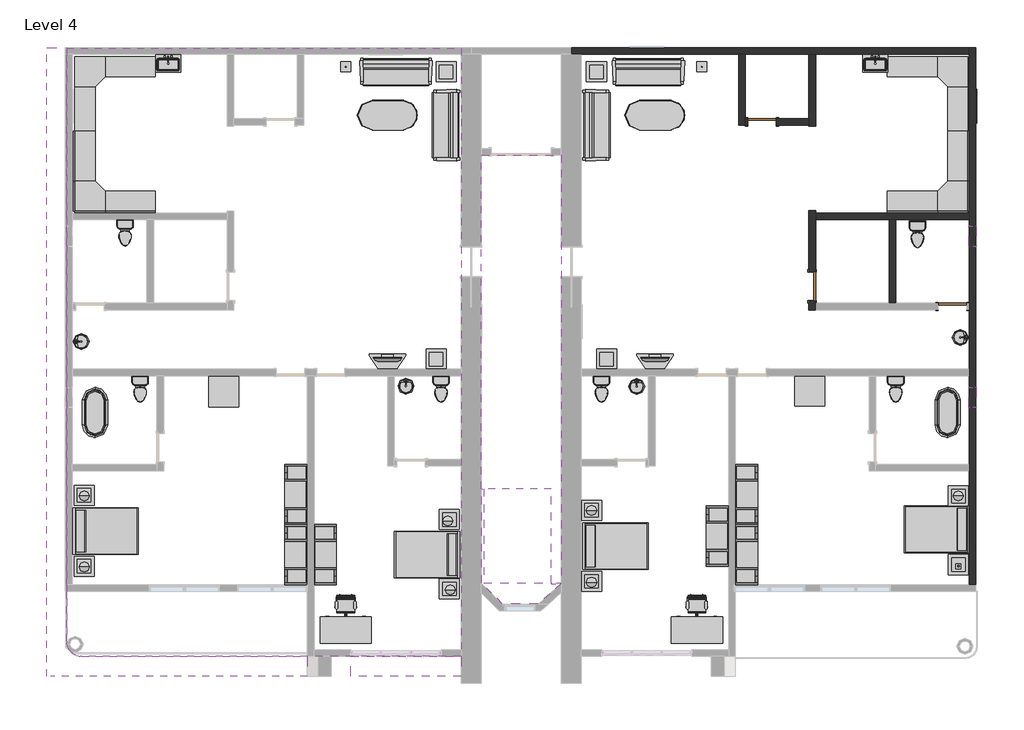
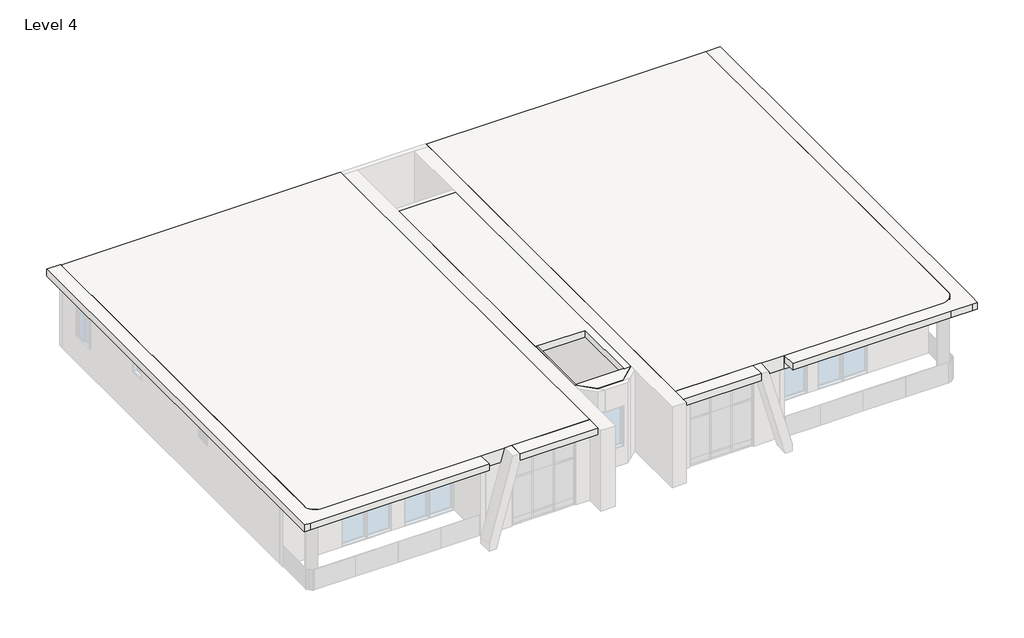
# One storey, part 3 of 3: 42 furniture elements, 14 flow terminals, 10 light fixtures, 8 walls, 5 slabs, 3 doors, 3 windows.
"""IFC4 building model written with IfcOpenShell, lengths in millimetres."""

from ifc_helpers import new_model, si_unit, point, frame, frame_2d, origin, place, context, project, spatial, polyline, circle_curve, trimmed, segment, composite_curve, outline, extrude, faceted_brep, transform, mapped, element, save
from components import door_2703ae13, door_10fd3a06, flow_terminal_38af2918, flow_terminal_d49f872f, toilet_domestic_3d_toilet_domestic_3d_f7549cf7, toilet_domestic_3d_toilet_domestic_3d_183bbd19, flow_terminal_b374fae2, furniture_07436f11, furniture_096e7f55, chair_task_arms_chair_task_arms_fa5a08ef, furniture_072f6425, furniture_cf0b6580, furniture_aff9b2fb, furniture_56245f3a, tv_stand_tv_stand_6ce107e5, furniture_b5c51a22, furniture_2c34a4f9, furniture_4d44e21c, furniture_45e3acac, light_fixture_100w_120v_8564026f, table_lamp_hemispheric_60w_120v_02721d88, window_0038ecf3, window_54100e87

model = new_model("IFC4")

# Units and contexts
model_context = context("Model", 3, world=origin())
ifc_project = project(units=[si_unit("LENGTHUNIT", "METRE", prefix="MILLI")], contexts=[model_context])

# Site, building, storey
site = spatial("IfcSite", under=ifc_project)
building = spatial("IfcBuilding", under=site)
storey = spatial("IfcBuildingStorey", under=building, Name="Level 4", Elevation=10972.8)

# Doors
placement = place(None, origin())
door_shape = door_2703ae13(model_context)
element("IfcDoor", 1, ObjectType="Door-Single-Panel.0001 : 34\" x 80\"", at=placement, inside=storey, context=model_context, shape_type="MappedRepresentation", body=[
    mapped(door_shape, transform((2522.0012296, 9464.0758558, 10972.8), x_axis=(-1.0, 0.0, 0.0), y_axis=(0.0, -1.0, 0.0), z_axis=(0.0, 0.0, 1.0))),
])
door_2_shape = door_10fd3a06(model_context)
element("IfcDoor", 2, ObjectType="Door-Single-Panel.0001 : 34\" x 80\"", at=placement, inside=storey, context=model_context, shape_type="MappedRepresentation", body=[
    mapped(door_2_shape, transform((8313.2012296, 3850.6758558, 10972.8), x_axis=(1.0, 0.0, 0.0), y_axis=(0.0, 1.0, 0.0), z_axis=(0.0, 0.0, 1.0))),
])
element("IfcDoor", 3, ObjectType="Door-Single-Panel.0001 : 34\" x 80\"", at=placement, inside=storey, context=model_context, shape_type="MappedRepresentation", body=[
    mapped(door_2_shape, transform((4046.0012296, 4460.2758558, 10972.8), x_axis=(0.0, -1.0, 0.0), y_axis=(1.0, 0.0, 0.0), z_axis=(0.0, 0.0, 1.0))),
])

# Flow terminals
flow_terminal_shape = flow_terminal_38af2918(model_context)
element("IfcFlowTerminal", 4, ObjectType="Sink Kitchen-Single : 30\" x 21\"", at=placement, inside=storey, context=model_context, shape_type="MappedRepresentation", body=[
    mapped(flow_terminal_shape, transform((-15540.388011, 11239.7304546, 10972.8), x_axis=(1.0, 0.0, 0.0), y_axis=(0.0, 1.0, 0.0), z_axis=(0.0, 0.0, 1.0))),
])
element("IfcFlowTerminal", 5, ObjectType="Sink Kitchen-Single : 30\" x 21\"", at=placement, inside=storey, context=model_context, shape_type="MappedRepresentation", body=[
    mapped(flow_terminal_shape, transform((5948.011989, 11239.7304546, 10972.8), x_axis=(1.0, 0.0, 0.0), y_axis=(0.0, 1.0, 0.0), z_axis=(0.0, 0.0, 1.0))),
])
flow_terminal_2_shape = flow_terminal_d49f872f(model_context)
element("IfcFlowTerminal", 6, ObjectType="Sink Vanity-Round : 19\" x 19\"", at=placement, inside=storey, context=model_context, shape_type="MappedRepresentation", body=[
    mapped(flow_terminal_2_shape, transform((-18084.6070794, 2687.2241152, 10972.8), x_axis=(0.0, 1.0, 0.0), y_axis=(-1.0, 0.0, 0.0), z_axis=(0.0, 0.0, 1.0))),
])
element("IfcFlowTerminal", 7, ObjectType="Sink Vanity-Round : 19\" x 19\"", at=placement, inside=storey, context=model_context, shape_type="MappedRepresentation", body=[
    mapped(flow_terminal_2_shape, transform((8462.2249463, 3007.5275963, 10972.8), x_axis=(0.0, -1.0, 0.0), y_axis=(1.0, 0.0, 0.0), z_axis=(0.0, 0.0, 1.0))),
])
element("IfcFlowTerminal", 8, ObjectType="Sink Vanity-Round : 19\" x 19\"", at=placement, inside=storey, context=model_context, shape_type="MappedRepresentation", body=[
    mapped(flow_terminal_2_shape, transform((-8395.050511, 1341.8921141, 10972.8), x_axis=(1.0, 0.0, 0.0), y_axis=(0.0, 1.0, 0.0), z_axis=(0.0, 0.0, 1.0))),
])
element("IfcFlowTerminal", 9, ObjectType="Sink Vanity-Round : 19\" x 19\"", at=placement, inside=storey, context=model_context, shape_type="MappedRepresentation", body=[
    mapped(flow_terminal_2_shape, transform((-1384.650511, 1331.0855344, 10972.8), x_axis=(1.0, 0.0, 0.0), y_axis=(0.0, 1.0, 0.0), z_axis=(0.0, 0.0, 1.0))),
])
toilet_domestic_3d_toilet_domestic_3d_shape = toilet_domestic_3d_toilet_domestic_3d_f7549cf7(model_context)
toilet_domestic_3d_toilet_domestic_3d_2_shape = toilet_domestic_3d_toilet_domestic_3d_183bbd19(model_context)
element("IfcFlowTerminal", 10, ObjectType="Toilet-Domestic-3D : Toilet-Domestic-3D", at=placement, inside=storey, context=model_context, shape_type="MappedRepresentation", body=[
    mapped(toilet_domestic_3d_toilet_domestic_3d_shape, transform((6586.0012296, 1247.7798284, 10972.8), x_axis=(1.0, 0.0, 0.0), y_axis=(0.0, 1.0, 0.0), z_axis=(0.0, 0.0, 1.0))),
    mapped(toilet_domestic_3d_toilet_domestic_3d_2_shape, transform((6586.0012296, 1247.7798284, 10972.8), x_axis=(1.0, 0.0, 0.0), y_axis=(0.0, 1.0, 0.0), z_axis=(0.0, 0.0, 1.0))),
])
element("IfcFlowTerminal", 11, ObjectType="Toilet-Domestic-3D : Toilet-Domestic-3D", at=placement, inside=storey, context=model_context, shape_type="MappedRepresentation", body=[
    mapped(toilet_domestic_3d_toilet_domestic_3d_shape, transform((-2354.7987704, 1247.7798284, 10972.8), x_axis=(1.0, 0.0, 0.0), y_axis=(0.0, 1.0, 0.0), z_axis=(0.0, 0.0, 1.0))),
    mapped(toilet_domestic_3d_toilet_domestic_3d_2_shape, transform((-2354.7987704, 1247.7798284, 10972.8), x_axis=(1.0, 0.0, 0.0), y_axis=(0.0, 1.0, 0.0), z_axis=(0.0, 0.0, 1.0))),
])
element("IfcFlowTerminal", 12, ObjectType="Toilet-Domestic-3D : Toilet-Domestic-3D", at=placement, inside=storey, context=model_context, shape_type="MappedRepresentation", body=[
    mapped(toilet_domestic_3d_toilet_domestic_3d_shape, transform((-16375.5987704, 1247.7798284, 10972.8), x_axis=(1.0, 0.0, 0.0), y_axis=(0.0, 1.0, 0.0), z_axis=(0.0, 0.0, 1.0))),
    mapped(toilet_domestic_3d_toilet_domestic_3d_2_shape, transform((-16375.5987704, 1247.7798284, 10972.8), x_axis=(1.0, 0.0, 0.0), y_axis=(0.0, 1.0, 0.0), z_axis=(0.0, 0.0, 1.0))),
])
element("IfcFlowTerminal", 13, ObjectType="Toilet-Domestic-3D : Toilet-Domestic-3D", at=placement, inside=storey, context=model_context, shape_type="MappedRepresentation", body=[
    mapped(toilet_domestic_3d_toilet_domestic_3d_shape, transform((-16832.7987704, 5997.5798284, 10972.8), x_axis=(1.0, 0.0, 0.0), y_axis=(0.0, 1.0, 0.0), z_axis=(0.0, 0.0, 1.0))),
    mapped(toilet_domestic_3d_toilet_domestic_3d_2_shape, transform((-16832.7987704, 5997.5798284, 10972.8), x_axis=(1.0, 0.0, 0.0), y_axis=(0.0, 1.0, 0.0), z_axis=(0.0, 0.0, 1.0))),
])
element("IfcFlowTerminal", 14, ObjectType="Toilet-Domestic-3D : Toilet-Domestic-3D", at=placement, inside=storey, context=model_context, shape_type="MappedRepresentation", body=[
    mapped(toilet_domestic_3d_toilet_domestic_3d_shape, transform((7246.4012296, 5946.7798284, 10972.8), x_axis=(1.0, 0.0, 0.0), y_axis=(0.0, 1.0, 0.0), z_axis=(0.0, 0.0, 1.0))),
    mapped(toilet_domestic_3d_toilet_domestic_3d_2_shape, transform((7246.4012296, 5946.7798284, 10972.8), x_axis=(1.0, 0.0, 0.0), y_axis=(0.0, 1.0, 0.0), z_axis=(0.0, 0.0, 1.0))),
])
element("IfcFlowTerminal", 15, ObjectType="Toilet-Domestic-3D : Toilet-Domestic-3D", at=placement, inside=storey, context=model_context, shape_type="MappedRepresentation", body=[
    mapped(toilet_domestic_3d_toilet_domestic_3d_shape, transform((-7231.5987704, 1247.7798284, 10972.8), x_axis=(1.0, 0.0, 0.0), y_axis=(0.0, 1.0, 0.0), z_axis=(0.0, 0.0, 1.0))),
    mapped(toilet_domestic_3d_toilet_domestic_3d_2_shape, transform((-7231.5987704, 1247.7798284, 10972.8), x_axis=(1.0, 0.0, 0.0), y_axis=(0.0, 1.0, 0.0), z_axis=(0.0, 0.0, 1.0))),
])
flow_terminal_3_shape = flow_terminal_b374fae2(model_context)
element("IfcFlowTerminal", 16, ObjectType="Tub-Free Standing-3D : 30\" x 60\"", at=placement, inside=storey, context=model_context, shape_type="MappedRepresentation", body=[
    mapped(flow_terminal_3_shape, transform((-17747.1987704, 624.8758558, 10972.8), x_axis=(1.0, 0.0, 0.0), y_axis=(0.0, 1.0, 0.0), z_axis=(0.0, 0.0, 1.0))),
])
element("IfcFlowTerminal", 17, ObjectType="Tub-Free Standing-3D : 30\" x 60\"", at=placement, inside=storey, context=model_context, shape_type="MappedRepresentation", body=[
    mapped(flow_terminal_3_shape, transform((8160.8012296, 624.8758558, 10972.8), x_axis=(1.0, 0.0, 0.0), y_axis=(0.0, 1.0, 0.0), z_axis=(0.0, 0.0, 1.0))),
])

# Furniture
furniture_shape = furniture_07436f11(model_context)
element("IfcFurniture", 18, ObjectType="96\" x 96\"", at=placement, inside=storey, context=model_context, shape_type="MappedRepresentation", body=[
    mapped(furniture_shape, transform((-18275.8670182, 11991.0988634, 10972.8), x_axis=(1.0, 0.0, 0.0), y_axis=(0.0, 1.0, 0.0), z_axis=(0.0, 0.0, 1.0))),
])
element("IfcFurniture", 19, ObjectType="96\" x 96\"", at=placement, inside=storey, context=model_context, shape_type="MappedRepresentation", body=[
    mapped(furniture_shape, transform((9316.2242372, 11364.3441035, 10972.8), x_axis=(0.0, -1.0, 0.0), y_axis=(1.0, 0.0, 0.0), z_axis=(0.0, 0.0, 1.0))),
])
furniture_2_shape = furniture_096e7f55(model_context)
element("IfcFurniture", 20, ObjectType="Bed-Shaker : Double 56\" x 78\"", at=placement, inside=storey, context=model_context, shape_type="MappedRepresentation", body=[
    mapped(furniture_2_shape, transform((-18407.5987704, -2962.8741442, 10972.8), x_axis=(0.0, 1.0, 0.0), y_axis=(-1.0, 0.0, 0.0), z_axis=(0.0, 0.0, 1.0))),
])
element("IfcFurniture", 21, ObjectType="Bed-Shaker : Double 56\" x 78\"", at=placement, inside=storey, context=model_context, shape_type="MappedRepresentation", body=[
    mapped(furniture_2_shape, transform((-6672.7987704, -3712.1741442, 10972.8), x_axis=(0.0, -1.0, 0.0), y_axis=(1.0, 0.0, 0.0), z_axis=(0.0, 0.0, 1.0))),
])
element("IfcFurniture", 22, ObjectType="Bed-Shaker : Double 56\" x 78\"", at=placement, inside=storey, context=model_context, shape_type="MappedRepresentation", body=[
    mapped(furniture_2_shape, transform((-2913.5987704, -3420.0741442, 10972.8), x_axis=(0.0, 1.0, 0.0), y_axis=(-1.0, 0.0, 0.0), z_axis=(0.0, 0.0, 1.0))),
])
element("IfcFurniture", 23, ObjectType="Bed-Shaker : Double 56\" x 78\"", at=placement, inside=storey, context=model_context, shape_type="MappedRepresentation", body=[
    mapped(furniture_2_shape, transform((8821.2012296, -2950.1741442, 10972.8), x_axis=(0.0, -1.0, 0.0), y_axis=(1.0, 0.0, 0.0), z_axis=(0.0, 0.0, 1.0))),
])
chair_task_arms_chair_task_arms_shape = chair_task_arms_chair_task_arms_fa5a08ef(model_context)
element("IfcFurniture", 24, ObjectType="Chair-Task Arms : Chair-Task Arms", at=placement, inside=storey, context=model_context, shape_type="MappedRepresentation", body=[
    mapped(chair_task_arms_chair_task_arms_shape, transform((681.7920493, -5184.3566833, 10972.8), x_axis=(-1.0, 0.0, 0.0), y_axis=(0.0, -1.0, 0.0), z_axis=(0.0, 0.0, 1.0))),
])
element("IfcFurniture", 25, ObjectType="Chair-Task Arms : Chair-Task Arms", at=placement, inside=storey, context=model_context, shape_type="MappedRepresentation", body=[
    mapped(chair_task_arms_chair_task_arms_shape, transform((-9986.2079507, -5184.3566833, 10972.8), x_axis=(-1.0, 0.0, 0.0), y_axis=(0.0, -1.0, 0.0), z_axis=(0.0, 0.0, 1.0))),
])
furniture_3_shape = furniture_072f6425(model_context)
element("IfcFurniture", 26, ObjectType="Desk : 60\" x 30\"", at=placement, inside=storey, context=model_context, shape_type="MappedRepresentation", body=[
    mapped(furniture_3_shape, transform((-10889.1987704, -6371.702585, 10972.8), x_axis=(1.0, 0.0, 0.0), y_axis=(0.0, 1.0, 0.0), z_axis=(0.0, 0.0, 1.0))),
])
element("IfcFurniture", 27, ObjectType="Desk : 60\" x 30\"", at=placement, inside=storey, context=model_context, shape_type="MappedRepresentation", body=[
    mapped(furniture_3_shape, transform((-221.1987704, -6371.702585, 10972.8), x_axis=(1.0, 0.0, 0.0), y_axis=(0.0, 1.0, 0.0), z_axis=(0.0, 0.0, 1.0))),
])
furniture_4_shape = furniture_cf0b6580(model_context)
element("IfcFurniture", 28, ObjectType="Entertainment Center : 72\" x 72\" x 24\"", at=placement, inside=storey, context=model_context, shape_type="MappedRepresentation", body=[
    mapped(furniture_4_shape, transform((1607.6012296, -3134.3241442, 10972.8), x_axis=(0.0, -1.0, 0.0), y_axis=(1.0, 0.0, 0.0), z_axis=(0.0, 0.0, 1.0))),
])
element("IfcFurniture", 29, ObjectType="Entertainment Center : 72\" x 72\" x 24\"", at=placement, inside=storey, context=model_context, shape_type="MappedRepresentation", body=[
    mapped(furniture_4_shape, transform((1607.6012296, -3693.1241442, 10972.8), x_axis=(0.0, 1.0, 0.0), y_axis=(-1.0, 0.0, 0.0), z_axis=(0.0, 0.0, 1.0))),
])
element("IfcFurniture", 30, ObjectType="Entertainment Center : 72\" x 72\" x 24\"", at=placement, inside=storey, context=model_context, shape_type="MappedRepresentation", body=[
    mapped(furniture_4_shape, transform((1607.6012296, -1864.3241442, 10972.8), x_axis=(0.0, 1.0, 0.0), y_axis=(-1.0, 0.0, 0.0), z_axis=(0.0, 0.0, 1.0))),
])
element("IfcFurniture", 31, ObjectType="Entertainment Center : 72\" x 72\" x 24\"", at=placement, inside=storey, context=model_context, shape_type="MappedRepresentation", body=[
    mapped(furniture_4_shape, transform((-11193.9987704, -3693.1241442, 10972.8), x_axis=(0.0, -1.0, 0.0), y_axis=(1.0, 0.0, 0.0), z_axis=(0.0, 0.0, 1.0))),
])
element("IfcFurniture", 32, ObjectType="Entertainment Center : 72\" x 72\" x 24\"", at=placement, inside=storey, context=model_context, shape_type="MappedRepresentation", body=[
    mapped(furniture_4_shape, transform((-11193.9987704, -1864.3241442, 10972.8), x_axis=(0.0, -1.0, 0.0), y_axis=(1.0, 0.0, 0.0), z_axis=(0.0, 0.0, 1.0))),
])
element("IfcFurniture", 33, ObjectType="Entertainment Center : 72\" x 72\" x 24\"", at=placement, inside=storey, context=model_context, shape_type="MappedRepresentation", body=[
    mapped(furniture_4_shape, transform((-11193.9987704, -3693.1241442, 10972.8), x_axis=(0.0, 1.0, 0.0), y_axis=(-1.0, 0.0, 0.0), z_axis=(0.0, 0.0, 1.0))),
])
furniture_5_shape = furniture_aff9b2fb(model_context)
element("IfcFurniture", 34, ObjectType="Sofa-Pensi : 84\"", at=placement, inside=storey, context=model_context, shape_type="MappedRepresentation", body=[
    mapped(furniture_5_shape, transform((-8881.8050204, 10710.9660197, 10972.8), x_axis=(1.0, 0.0, 0.0), y_axis=(0.0, 1.0, 0.0), z_axis=(0.0, 0.0, 1.0))),
])
element("IfcFurniture", 35, ObjectType="Sofa-Pensi : 84\"", at=placement, inside=storey, context=model_context, shape_type="MappedRepresentation", body=[
    mapped(furniture_5_shape, transform((-7356.3086065, 9641.0821058, 10972.8), x_axis=(0.0, -1.0, 0.0), y_axis=(1.0, 0.0, 0.0), z_axis=(0.0, 0.0, 1.0))),
])
element("IfcFurniture", 36, ObjectType="Sofa-Pensi : 84\"", at=placement, inside=storey, context=model_context, shape_type="MappedRepresentation", body=[
    mapped(furniture_5_shape, transform((-2230.0889343, 9083.8696058, 10972.8), x_axis=(0.0, 1.0, 0.0), y_axis=(-1.0, 0.0, 0.0), z_axis=(0.0, 0.0, 1.0))),
])
element("IfcFurniture", 37, ObjectType="Sofa-Pensi : 84\"", at=placement, inside=storey, context=model_context, shape_type="MappedRepresentation", body=[
    mapped(furniture_5_shape, transform((-1211.0050204, 10710.9660197, 10972.8), x_axis=(1.0, 0.0, 0.0), y_axis=(0.0, 1.0, 0.0), z_axis=(0.0, 0.0, 1.0))),
])
furniture_6_shape = furniture_56245f3a(model_context)
element("IfcFurniture", 38, ObjectType="TV - Flat Screen : 32\"", at=placement, inside=storey, context=model_context, shape_type="MappedRepresentation", body=[
    mapped(furniture_6_shape, transform((-8861.1432846, 2232.8144794, 11887.2), x_axis=(-1.0, 0.0, 0.0), y_axis=(0.0, -1.0, 0.0), z_axis=(0.0, 0.0, 1.0))),
])
element("IfcFurniture", 39, ObjectType="TV - Flat Screen : 32\"", at=placement, inside=storey, context=model_context, shape_type="MappedRepresentation", body=[
    mapped(furniture_6_shape, transform((-733.1432846, 2232.8144794, 11887.2), x_axis=(-1.0, 0.0, 0.0), y_axis=(0.0, -1.0, 0.0), z_axis=(0.0, 0.0, 1.0))),
])
tv_stand_tv_stand_shape = tv_stand_tv_stand_6ce107e5(model_context)
element("IfcFurniture", 40, ObjectType="TV Stand : TV Stand", at=placement, inside=storey, context=model_context, shape_type="MappedRepresentation", body=[
    mapped(tv_stand_tv_stand_shape, transform((-8732.0107683, 1945.6758558, 10972.8), x_axis=(-1.0, 0.0, 0.0), y_axis=(0.0, -1.0, 0.0), z_axis=(0.0, 0.0, 1.0))),
])
element("IfcFurniture", 41, ObjectType="TV Stand : TV Stand", at=placement, inside=storey, context=model_context, shape_type="MappedRepresentation", body=[
    mapped(tv_stand_tv_stand_shape, transform((-604.0107683, 1945.6758558, 10972.8), x_axis=(-1.0, 0.0, 0.0), y_axis=(0.0, -1.0, 0.0), z_axis=(0.0, 0.0, 1.0))),
])
furniture_7_shape = furniture_b5c51a22(model_context)
element("IfcFurniture", 42, ObjectType="Table-Coffee : 24\" x 24\" x 24\"", at=placement, inside=storey, context=model_context, shape_type="MappedRepresentation", body=[
    mapped(furniture_7_shape, transform((-7097.4645371, 10892.864778, 10972.8), x_axis=(1.0, 0.0, 0.0), y_axis=(0.0, 1.0, 0.0), z_axis=(0.0, 0.0, 1.0))),
])
element("IfcFurniture", 43, ObjectType="Table-Coffee : 24\" x 24\" x 24\"", at=placement, inside=storey, context=model_context, shape_type="MappedRepresentation", body=[
    mapped(furniture_7_shape, transform((-2525.4645371, 10892.864778, 10972.8), x_axis=(1.0, 0.0, 0.0), y_axis=(0.0, 1.0, 0.0), z_axis=(0.0, 0.0, 1.0))),
])
element("IfcFurniture", 44, ObjectType="Table-Coffee : 24\" x 24\" x 24\"", at=placement, inside=storey, context=model_context, shape_type="MappedRepresentation", body=[
    mapped(furniture_7_shape, transform((-7402.2645371, 2155.264778, 10972.8), x_axis=(1.0, 0.0, 0.0), y_axis=(0.0, 1.0, 0.0), z_axis=(0.0, 0.0, 1.0))),
])
element("IfcFurniture", 45, ObjectType="Table-Coffee : 24\" x 24\" x 24\"", at=placement, inside=storey, context=model_context, shape_type="MappedRepresentation", body=[
    mapped(furniture_7_shape, transform((-2220.6645371, 2155.264778, 10972.8), x_axis=(1.0, 0.0, 0.0), y_axis=(0.0, 1.0, 0.0), z_axis=(0.0, 0.0, 1.0))),
])
element("IfcFurniture", 46, ObjectType="Table-Coffee : 24\" x 24\" x 24\"", at=placement, inside=storey, context=model_context, shape_type="MappedRepresentation", body=[
    mapped(furniture_7_shape, transform((-2677.8645371, -4601.135222, 10972.8), x_axis=(1.0, 0.0, 0.0), y_axis=(0.0, 1.0, 0.0), z_axis=(0.0, 0.0, 1.0))),
])
element("IfcFurniture", 47, ObjectType="Table-Coffee : 24\" x 24\" x 24\"", at=placement, inside=storey, context=model_context, shape_type="MappedRepresentation", body=[
    mapped(furniture_7_shape, transform((-18095.6645371, -4143.935222, 10972.8), x_axis=(1.0, 0.0, 0.0), y_axis=(0.0, 1.0, 0.0), z_axis=(0.0, 0.0, 1.0))),
])
element("IfcFurniture", 48, ObjectType="Table-Coffee : 24\" x 24\" x 24\"", at=placement, inside=storey, context=model_context, shape_type="MappedRepresentation", body=[
    mapped(furniture_7_shape, transform((-18095.6645371, -1984.935222, 10972.8), x_axis=(1.0, 0.0, 0.0), y_axis=(0.0, 1.0, 0.0), z_axis=(0.0, 0.0, 1.0))),
])
element("IfcFurniture", 49, ObjectType="Table-Coffee : 24\" x 24\" x 24\"", at=placement, inside=storey, context=model_context, shape_type="MappedRepresentation", body=[
    mapped(furniture_7_shape, transform((-2677.8645371, -2442.135222, 10972.8), x_axis=(1.0, 0.0, 0.0), y_axis=(0.0, 1.0, 0.0), z_axis=(0.0, 0.0, 1.0))),
])
element("IfcFurniture", 50, ObjectType="Table-Coffee : 24\" x 24\" x 24\"", at=placement, inside=storey, context=model_context, shape_type="MappedRepresentation", body=[
    mapped(furniture_7_shape, transform((8472.7354629, -4093.135222, 10972.8), x_axis=(1.0, 0.0, 0.0), y_axis=(0.0, 1.0, 0.0), z_axis=(0.0, 0.0, 1.0))),
])
element("IfcFurniture", 51, ObjectType="Table-Coffee : 24\" x 24\" x 24\"", at=placement, inside=storey, context=model_context, shape_type="MappedRepresentation", body=[
    mapped(furniture_7_shape, transform((8472.7354629, -2010.335222, 10972.8), x_axis=(1.0, 0.0, 0.0), y_axis=(0.0, 1.0, 0.0), z_axis=(0.0, 0.0, 1.0))),
])
element("IfcFurniture", 52, ObjectType="Table-Coffee : 24\" x 24\" x 24\"", at=placement, inside=storey, context=model_context, shape_type="MappedRepresentation", body=[
    mapped(furniture_7_shape, transform((-6995.8645371, -4832.0414601, 10972.8), x_axis=(1.0, 0.0, 0.0), y_axis=(0.0, 1.0, 0.0), z_axis=(0.0, 0.0, 1.0))),
])
element("IfcFurniture", 53, ObjectType="Table-Coffee : 24\" x 24\" x 24\"", at=placement, inside=storey, context=model_context, shape_type="MappedRepresentation", body=[
    mapped(furniture_7_shape, transform((-6995.8645371, -2723.8414601, 10972.8), x_axis=(1.0, 0.0, 0.0), y_axis=(0.0, 1.0, 0.0), z_axis=(0.0, 0.0, 1.0))),
])
furniture_8_shape = furniture_2c34a4f9(model_context)
element("IfcFurniture", 54, ObjectType="Table-Dining Oval : 36\" x 72\"", at=placement, inside=storey, context=model_context, shape_type="MappedRepresentation", body=[
    mapped(furniture_8_shape, transform((-8455.3790983, 10025.3742164, 10972.8), x_axis=(1.0, 0.0, 0.0), y_axis=(0.0, 1.0, 0.0), z_axis=(0.0, 0.0, 1.0))),
])
element("IfcFurniture", 55, ObjectType="Table-Dining Oval : 36\" x 72\"", at=placement, inside=storey, context=model_context, shape_type="MappedRepresentation", body=[
    mapped(furniture_8_shape, transform((-327.3790983, 10025.3742164, 10972.8), x_axis=(1.0, 0.0, 0.0), y_axis=(0.0, 1.0, 0.0), z_axis=(0.0, 0.0, 1.0))),
])
furniture_9_shape = furniture_4d44e21c(model_context)
element("IfcFurniture", 56, ObjectType="Table-Rectangular : 36\" x 36\"", at=placement, inside=storey, context=model_context, shape_type="MappedRepresentation", body=[
    mapped(furniture_9_shape, transform((-13835.5987704, 1259.8758558, 10972.8), x_axis=(1.0, 0.0, 0.0), y_axis=(0.0, 1.0, 0.0), z_axis=(0.0, 0.0, 1.0))),
])
element("IfcFurniture", 57, ObjectType="Table-Rectangular : 36\" x 36\"", at=placement, inside=storey, context=model_context, shape_type="MappedRepresentation", body=[
    mapped(furniture_9_shape, transform((3969.8012296, 1285.2758558, 10972.8), x_axis=(1.0, 0.0, 0.0), y_axis=(0.0, 1.0, 0.0), z_axis=(0.0, 0.0, 1.0))),
])
furniture_10_shape = furniture_45e3acac(model_context)
element("IfcFurniture", 58, ObjectType="Work Station Cubicle : 96\" x 96\"", at=placement, inside=storey, context=model_context, shape_type="MappedRepresentation", body=[
    mapped(furniture_10_shape, transform((-18902.621778, 6827.207608, 10972.8), x_axis=(0.0, 1.0, 0.0), y_axis=(-1.0, 0.0, 0.0), z_axis=(0.0, 0.0, 1.0))),
])
element("IfcFurniture", 59, ObjectType="Work Station Cubicle : 96\" x 96\"", at=placement, inside=storey, context=model_context, shape_type="MappedRepresentation", body=[
    mapped(furniture_10_shape, transform((8689.4694774, 6200.4528481, 10972.8), x_axis=(-1.0, 0.0, 0.0), y_axis=(0.0, -1.0, 0.0), z_axis=(0.0, 0.0, 1.0))),
])

# Light fixtures
light_fixture_100w_120v_shape = light_fixture_100w_120v_8564026f(model_context)
element("IfcLightFixture", 60, ObjectType="100W - 120V", at=placement, inside=storey, context=model_context, shape_type="MappedRepresentation", body=[
    mapped(light_fixture_100w_120v_shape, transform((-10127.1987704, 11140.4758558, 10972.8), x_axis=(1.0, 0.0, 0.0), y_axis=(0.0, 1.0, 0.0), z_axis=(0.0, 0.0, 1.0))),
])
element("IfcLightFixture", 61, ObjectType="100W - 120V", at=placement, inside=storey, context=model_context, shape_type="MappedRepresentation", body=[
    mapped(light_fixture_100w_120v_shape, transform((693.2012296, 11140.4758558, 10972.8), x_axis=(1.0, 0.0, 0.0), y_axis=(0.0, 1.0, 0.0), z_axis=(0.0, 0.0, 1.0))),
])
table_lamp_hemispheric_60w_120v_shape = table_lamp_hemispheric_60w_120v_02721d88(model_context)
element("IfcLightFixture", 62, ObjectType="Table Lamp - Hemispheric : 60W - 120V", at=placement, inside=storey, context=model_context, shape_type="MappedRepresentation", body=[
    mapped(table_lamp_hemispheric_60w_120v_shape, transform((-18077.3987704, -1915.1241442, 11582.4), x_axis=(1.0, 0.0, 0.0), y_axis=(0.0, 1.0, 0.0), z_axis=(0.0, 0.0, 1.0))),
])
element("IfcLightFixture", 63, ObjectType="Table Lamp - Hemispheric : 60W - 120V", at=placement, inside=storey, context=model_context, shape_type="MappedRepresentation", body=[
    mapped(table_lamp_hemispheric_60w_120v_shape, transform((-7028.3987704, -2666.7303823, 11582.4), x_axis=(1.0, 0.0, 0.0), y_axis=(0.0, 1.0, 0.0), z_axis=(0.0, 0.0, 1.0))),
])
element("IfcLightFixture", 64, ObjectType="Table Lamp - Hemispheric : 60W - 120V", at=placement, inside=storey, context=model_context, shape_type="MappedRepresentation", body=[
    mapped(table_lamp_hemispheric_60w_120v_shape, transform((-2659.5987704, -2346.9241442, 11582.4), x_axis=(1.0, 0.0, 0.0), y_axis=(0.0, 1.0, 0.0), z_axis=(0.0, 0.0, 1.0))),
])
element("IfcLightFixture", 65, ObjectType="Table Lamp - Hemispheric : 60W - 120V", at=placement, inside=storey, context=model_context, shape_type="MappedRepresentation", body=[
    mapped(table_lamp_hemispheric_60w_120v_shape, transform((8491.0012296, -4048.7241442, 11887.2), x_axis=(1.0, 0.0, 0.0), y_axis=(0.0, 1.0, 0.0), z_axis=(0.0, 0.0, 1.0))),
])
element("IfcLightFixture", 66, ObjectType="Table Lamp - Hemispheric : 60W - 120V", at=placement, inside=storey, context=model_context, shape_type="MappedRepresentation", body=[
    mapped(table_lamp_hemispheric_60w_120v_shape, transform((8491.0012296, -1915.1241442, 11582.4), x_axis=(1.0, 0.0, 0.0), y_axis=(0.0, 1.0, 0.0), z_axis=(0.0, 0.0, 1.0))),
])
element("IfcLightFixture", 67, ObjectType="Table Lamp - Hemispheric : 60W - 120V", at=placement, inside=storey, context=model_context, shape_type="MappedRepresentation", body=[
    mapped(table_lamp_hemispheric_60w_120v_shape, transform((-2659.5987704, -4531.3241442, 11582.4), x_axis=(1.0, 0.0, 0.0), y_axis=(0.0, 1.0, 0.0), z_axis=(0.0, 0.0, 1.0))),
])
element("IfcLightFixture", 68, ObjectType="Table Lamp - Hemispheric : 60W - 120V", at=placement, inside=storey, context=model_context, shape_type="MappedRepresentation", body=[
    mapped(table_lamp_hemispheric_60w_120v_shape, transform((-6952.1987704, -4762.2303823, 11582.4), x_axis=(1.0, 0.0, 0.0), y_axis=(0.0, 1.0, 0.0), z_axis=(0.0, 0.0, 1.0))),
])
element("IfcLightFixture", 69, ObjectType="Table Lamp - Hemispheric : 60W - 120V", at=placement, inside=storey, context=model_context, shape_type="MappedRepresentation", body=[
    mapped(table_lamp_hemispheric_60w_120v_shape, transform((-18077.3987704, -4074.1241442, 11582.4), x_axis=(1.0, 0.0, 0.0), y_axis=(0.0, 1.0, 0.0), z_axis=(0.0, 0.0, 1.0))),
])

# Slabs
element("IfcSlab", 70, ObjectType="Generic - 12\" cream", at=placement, inside=storey, context=model_context, shape_type="SweptSolid", body=[
    extrude(outline(composite_curve([segment(polyline([(-6621.9987704, 11699.2758558), (-6621.9987704, -6791.9241442), (-11295.5987704, -6791.9241442), (-18153.5987704, -6791.9241442)]), True, "CONTINUOUS"), segment(trimmed(circle_curve(frame_2d((-18153.5987704, -6334.7241442)), 457.2), [point((-18153.5987704, -6791.9241442))], [point((-18610.7987704, -6334.7241442))], False, "CARTESIAN"), True, "CONTINUOUS"), segment(polyline([(-18610.7987704, -6334.7241442), (-18610.7987704, 11699.2758558), (-6621.9987704, 11699.2758558)]), True, "CONTINUOUS")], self_intersect=False)), frame((0.0, 0.0, 14020.8), z_axis=(0.0, 0.0, 1.0), x_axis=(1.0, 0.0, 0.0)), (0.0, 0.0, 1.0), 609.6),
    extrude(outline(composite_curve([segment(trimmed(circle_curve(frame_2d((8511.8043381, -6277.3874522)), 514.536692), [point((9024.4012296, -6322.0241442))], [point((8511.8043381, -6791.9241442))], False, "CARTESIAN"), True, "CONTINUOUS"), segment(polyline([(8511.8043381, -6791.9241442), (1709.2012296, -6791.9241442), (-2862.7987704, -6791.9241442), (-2964.3987704, -6791.9241442), (-2964.3987704, 11699.2758558), (9024.4012296, 11699.2758558), (9024.4012296, -6322.0241442)]), True, "CONTINUOUS")], self_intersect=False)), frame((0.0, 0.0, 14020.8), z_axis=(0.0, 0.0, 1.0), x_axis=(1.0, 0.0, 0.0)), (0.0, 0.0, 1.0), 609.6),
])
element("IfcSlab", 71, ObjectType="Generic - 12\" white", at=placement, inside=storey, context=model_context, shape_type="SweptSolid", body=[
    extrude(outline(composite_curve([segment(polyline([(9634.0012296, 11699.2758558), (9634.0012296, -6931.6241442), (9634.0012296, -7401.5241442), (9430.8012296, -7401.5241442), (8511.8043381, -7401.5241442), (1709.2012296, -7401.5241442), (1709.2012296, -6791.9241442), (8511.8043381, -6791.9241442)]), True, "CONTINUOUS"), segment(trimmed(circle_curve(frame_2d((8511.8043381, -6277.3874522)), 514.536692), [point((8511.8043381, -6791.9241442))], [point((9024.4012296, -6322.0241442))], True, "CARTESIAN"), True, "CONTINUOUS"), segment(polyline([(9024.4012296, -6322.0241442), (9024.4012296, 11699.2758558), (9634.0012296, 11699.2758558)]), True, "CONTINUOUS")], self_intersect=False)), frame((0.0, 0.0, 14325.6), z_axis=(0.0, 0.0, 1.0), x_axis=(1.0, 0.0, 0.0)), (0.0, 0.0, 1.0), 304.8),
    extrude(outline(composite_curve([segment(polyline([(-18610.7987704, 11724.6758558), (-18610.7987704, -6334.7241442)]), True, "CONTINUOUS"), segment(trimmed(circle_curve(frame_2d((-18153.5987704, -6334.7241442)), 457.2), [point((-18610.7987704, -6334.7241442))], [point((-18153.5987704, -6791.9241442))], True, "CARTESIAN"), True, "CONTINUOUS"), segment(polyline([(-18153.5987704, -6791.9241442), (-11295.5987704, -6791.9241442), (-11295.5987704, -7401.5241442), (-18966.3987704, -7401.5241442), (-19220.3987704, -7401.5241442), (-19220.3987704, 11724.6758558), (-18610.7987704, 11724.6758558)]), True, "CONTINUOUS")], self_intersect=False)), frame((0.0, 0.0, 14325.6), z_axis=(0.0, 0.0, 1.0), x_axis=(1.0, 0.0, 0.0)), (0.0, 0.0, 1.0), 304.8),
])
element("IfcSlab", 72, ObjectType="Generic - 12\" white", at=placement, inside=storey, context=model_context, shape_type="SweptSolid", body=[
    extrude(outline(polyline([(385.6468143, -6791.9241442), (385.6468143, -7401.5241442), (-2964.3987704, -7401.5241442), (-2964.3987704, -6791.9241442), (385.6468143, -6791.9241442)])), frame((0.0, 0.0, 14325.6), z_axis=(0.0, 0.0, 1.0), x_axis=(1.0, 0.0, 0.0)), (0.0, 0.0, 1.0), 304.8),
    extrude(outline(polyline([(-9974.7987704, -6791.9241442), (-6621.9987704, -6791.9241442), (-6621.9987704, -7401.5241442), (-9974.7987704, -7401.5241442), (-9974.7987704, -6791.9241442)])), frame((0.0, 0.0, 14325.6), z_axis=(0.0, 0.0, 1.0), x_axis=(1.0, 0.0, 0.0)), (0.0, 0.0, 1.0), 304.8),
])
element("IfcSlab", 73, ObjectType="Generic - 12\" white", at=placement, inside=storey, context=model_context, shape_type="SweptSolid", body=[
    extrude(outline(polyline([(-3573.9987704, 8448.0758558), (-3573.9987704, -1691.5549149), (-3573.9987704, -4572.9908503), (-3878.7987704, -4572.9908503), (-3878.7987704, -1691.5549149), (-6012.3987704, -1691.5549149), (-6012.3987704, 8448.0758558), (-3573.9987704, 8448.0758558)])), frame((0.0, 0.0, 14325.6), z_axis=(0.0, 0.0, 1.0), x_axis=(1.0, 0.0, 0.0)), (0.0, 0.0, 1.0), 304.8),
])
element("IfcSlab", 74, ObjectType="Generic - 12\" white", at=placement, inside=storey, context=model_context, shape_type="SweptSolid", body=[
    extrude(outline(polyline([(-5940.8822214, -1691.5549149), (-5940.8822214, -4554.2130548), (-3883.4822214, -4554.2130548), (-3883.4822214, -4579.6130548), (-3594.7153195, -4579.6130548), (-4277.1570449, -5188.2185522), (-5369.3570449, -5188.2185522), (-5997.9749734, -4559.6006237), (-5997.9749734, -1691.5549149), (-5940.8822214, -1691.5549149)])), frame((0.0, 0.0, 14325.6), z_axis=(0.0, 0.0, 1.0), x_axis=(1.0, 0.0, 0.0)), (0.0, 0.0, 1.0), 304.8),
])

# Walls
element("IfcWall", 75, ObjectType="Generic - 8\" cream", at=placement, inside=storey, context=model_context, shape_type="Brep", body=[
    faceted_brep([(8821.2012296, 11724.6758558, 10972.8), (8821.2012296, 11521.4758558, 10972.8), (8821.2012296, 6695.4758558, 10972.8), (8821.2012296, 6492.2758558, 10972.8), (8821.2012296, 3952.2758558, 10972.8), (8821.2012296, 3749.0758558, 10972.8), (8821.2012296, 1945.6758558, 10972.8), (8821.2012296, 1742.4758558, 10972.8), (8821.2012296, -949.9241442, 10972.8), (8821.2012296, -1153.1241442, 10972.8), (8821.2012296, -4607.5241442, 10972.8), (8821.2012296, -4607.5241442, 14020.8), (8821.2012296, -1153.1241442, 14020.8), (8821.2012296, -949.9241442, 14020.8), (8821.2012296, 1742.4758558, 14020.8), (8821.2012296, 1945.6758558, 14020.8), (8821.2012296, 3749.0758558, 14020.8), (8821.2012296, 3952.2758558, 14020.8), (8821.2012296, 6492.2758558, 14020.8), (8821.2012296, 6695.4758558, 14020.8), (8821.2012296, 11521.4758558, 14020.8), (8821.2012296, 11724.6758558, 14020.8), (8821.2012296, 10403.8758558, 12192.0), (8821.2012296, 10403.8758558, 13411.2), (8821.2012296, 9489.4758558, 13411.2), (8821.2012296, 9489.4758558, 12192.0), (8821.2012296, 777.2758558, 13716.0), (8821.2012296, 777.2758558, 13106.4), (8821.2012296, 1386.8758558, 13106.4), (8821.2012296, 1386.8758558, 13716.0), (8821.2012296, 6289.0758558, 13106.4), (8821.2012296, 6289.0758558, 13716.0), (8821.2012296, 5679.4758558, 13716.0), (8821.2012296, 5679.4758558, 13106.4), (9024.4012296, -4607.5241442, 10972.8), (9024.4012296, 11724.6758558, 10972.8), (9024.4012296, 11724.6758558, 14020.8), (9024.4012296, -4607.5241442, 14020.8), (9024.4012296, 10403.8758558, 13411.2), (9024.4012296, 10403.8758558, 12192.0), (9024.4012296, 9489.4758558, 12192.0), (9024.4012296, 9489.4758558, 13411.2), (9024.4012296, 777.2758558, 13106.4), (9024.4012296, 777.2758558, 13716.0), (9024.4012296, 1386.8758558, 13716.0), (9024.4012296, 1386.8758558, 13106.4), (9024.4012296, 6289.0758558, 13716.0), (9024.4012296, 6289.0758558, 13106.4), (9024.4012296, 5679.4758558, 13106.4), (9024.4012296, 5679.4758558, 13716.0)], [[[0, 1, 2, 3, 4, 5, 6, 7, 8, 9, 10, 11, 12, 13, 14, 15, 16, 17, 18, 19, 20, 21], [22, 23, 24, 25], [26, 27, 28, 29], [30, 31, 32, 33]], [[34, 35, 36, 37], [38, 39, 40, 41], [42, 43, 44, 45], [46, 47, 48, 49]], [[10, 9, 8, 7, 6, 5, 4, 3, 2, 1, 0, 35, 34]], [[21, 20, 19, 18, 17, 16, 15, 14, 13, 12, 11, 37, 36]], [[0, 21, 36, 35]], [[11, 10, 34, 37]], [[39, 38, 23, 22]], [[40, 39, 22, 25]], [[41, 40, 25, 24]], [[38, 41, 24, 23]], [[26, 43, 42, 27]], [[27, 42, 45, 28]], [[28, 45, 44, 29]], [[43, 26, 29, 44]], [[46, 31, 30, 47]], [[47, 30, 33, 48]], [[48, 33, 32, 49]], [[31, 46, 49, 32]]]),
])
element("IfcWall", 76, ObjectType="Generic - 8\" cream", at=placement, inside=storey, context=model_context, shape_type="Brep", body=[
    faceted_brep([(3944.4012296, 11521.4758558, 10972.8), (3944.4012296, 9565.6758558, 10972.8), (3944.4012296, 9362.4758558, 10972.8), (3944.4012296, 9337.0758558, 10972.8), (3944.4012296, 9337.0758558, 14020.8), (3944.4012296, 9362.4758558, 14020.8), (3944.4012296, 9565.6758558, 14020.8), (3944.4012296, 11521.4758558, 14020.8), (4147.6012296, 11521.4758558, 10972.8), (4147.6012296, 11521.4758558, 14020.8), (4147.6012296, 9337.0758558, 14020.8), (4147.6012296, 9337.0758558, 10972.8)], [[[0, 1, 2, 3, 4, 5, 6, 7]], [[8, 9, 10, 11]], [[3, 2, 1, 0, 8, 11]], [[4, 3, 11, 10]], [[7, 6, 5, 4, 10, 9]], [[0, 7, 9, 8]]]),
])
element("IfcWall", 77, ObjectType="Generic - 8\" cream", at=placement, inside=storey, context=model_context, shape_type="Brep", body=[
    faceted_brep([(4147.6012296, 6492.2758558, 10972.8), (6382.8012296, 6492.2758558, 10972.8), (6586.0012296, 6492.2758558, 10972.8), (8821.2012296, 6492.2758558, 10972.8), (8821.2012296, 6492.2758558, 14020.8), (6586.0012296, 6492.2758558, 14020.8), (6382.8012296, 6492.2758558, 14020.8), (4147.6012296, 6492.2758558, 14020.8), (4147.6012296, 6695.4758558, 10972.8), (4147.6012296, 6695.4758558, 14020.8), (8821.2012296, 6695.4758558, 14020.8), (8821.2012296, 6695.4758558, 10972.8)], [[[0, 1, 2, 3, 4, 5, 6, 7]], [[8, 9, 10, 11]], [[3, 2, 1, 0, 8, 11]], [[7, 6, 5, 4, 10, 9]], [[0, 7, 9, 8]], [[4, 3, 11, 10]]]),
])
element("IfcWall", 78, ObjectType="Generic - 8\" cream", at=placement, inside=storey, context=model_context, shape_type="SweptSolid", body=[
    extrude(outline(polyline([(14020.8, 3944.4012296), (14020.8, 2014.0012296), (10972.8, 2014.0012296), (10972.8, 2090.2012296), (13004.8, 2090.2012296), (13004.8, 2953.8012296), (10972.8, 2953.8012296), (10972.8, 3944.4012296), (14020.8, 3944.4012296)])), frame((0.0, 9362.4758558, 0.0), z_axis=(0.0, 1.0, 0.0), x_axis=(0.0, 0.0, 1.0)), (0.0, 0.0, 1.0), 203.2),
])
element("IfcWall", 79, ObjectType="Generic - 8\" cream", at=placement, inside=storey, context=model_context, shape_type="SweptSolid", body=[
    extrude(outline(polyline([(6382.8012296, 3952.2758558), (6382.8012296, 6492.2758558), (6586.0012296, 6492.2758558), (6586.0012296, 3952.2758558), (6382.8012296, 3952.2758558)])), frame((0.0, 0.0, 10972.8), z_axis=(0.0, 0.0, 1.0), x_axis=(1.0, 0.0, 0.0)), (0.0, 0.0, 1.0), 3048.0),
])
element("IfcWall", 80, ObjectType="Generic - 8\" cream", at=placement, inside=storey, context=model_context, shape_type="Brep", body=[
    faceted_brep([(3944.4012296, 3749.0758558, 14020.8), (3944.4012296, 6771.6758558, 14020.8), (3944.4012296, 6771.6758558, 10972.8), (3944.4012296, 4892.0758558, 10972.8), (3944.4012296, 4892.0758558, 13004.8), (3944.4012296, 4028.4758558, 13004.8), (3944.4012296, 4028.4758558, 10972.8), (3944.4012296, 3749.0758558, 10972.8), (4147.6012296, 6771.6758558, 14020.8), (4147.6012296, 6695.4758558, 14020.8), (4147.6012296, 6492.2758558, 14020.8), (4147.6012296, 3952.2758558, 14020.8), (4147.6012296, 3749.0758558, 14020.8), (4147.6012296, 3749.0758558, 10972.8), (4147.6012296, 3952.2758558, 10972.8), (4147.6012296, 4028.4758558, 10972.8), (4147.6012296, 4028.4758558, 13004.8), (4147.6012296, 4892.0758558, 13004.8), (4147.6012296, 4892.0758558, 10972.8), (4147.6012296, 6492.2758558, 10972.8), (4147.6012296, 6695.4758558, 10972.8), (4147.6012296, 6771.6758558, 10972.8)], [[[0, 1, 2, 3, 4, 5, 6, 7]], [[8, 9, 10, 11, 12, 13, 14, 15, 16, 17, 18, 19, 20, 21]], [[2, 21, 20, 19, 18, 3]], [[13, 7, 6, 15, 14]], [[1, 0, 12, 11, 10, 9, 8]], [[2, 1, 8, 21]], [[0, 7, 13, 12]], [[5, 16, 15, 6]], [[16, 5, 4, 17]], [[17, 4, 3, 18]]]),
])
element("IfcWall", 81, ObjectType="Generic - 8\" cream", at=placement, inside=storey, context=model_context, shape_type="Brep", body=[
    faceted_brep([(-3269.1987704, 11521.4758558, 10972.8), (-2964.3987704, 11521.4758558, 10972.8), (1810.8012296, 11521.4758558, 10972.8), (2014.0012296, 11521.4758558, 10972.8), (3944.4012296, 11521.4758558, 10972.8), (4147.6012296, 11521.4758558, 10972.8), (8821.2012296, 11521.4758558, 10972.8), (8821.2012296, 11521.4758558, 14020.8), (4147.6012296, 11521.4758558, 14020.8), (3944.4012296, 11521.4758558, 14020.8), (2014.0012296, 11521.4758558, 14020.8), (1810.8012296, 11521.4758558, 14020.8), (-2964.3987704, 11521.4758558, 14020.8), (-3269.1987704, 11521.4758558, 14020.8), (-1440.3987704, 11521.4758558, 13411.2), (-525.9987704, 11521.4758558, 13411.2), (-525.9987704, 11521.4758558, 12192.0), (-1440.3987704, 11521.4758558, 12192.0), (-3269.1987704, 11724.6758558, 10972.8), (-3269.1987704, 11724.6758558, 14020.8), (-2964.3987704, 11724.6758558, 14020.8), (8821.2012296, 11724.6758558, 14020.8), (8821.2012296, 11724.6758558, 10972.8), (-1440.3987704, 11724.6758558, 13411.2), (-1440.3987704, 11724.6758558, 12192.0), (-525.9987704, 11724.6758558, 12192.0), (-525.9987704, 11724.6758558, 13411.2)], [[[0, 1, 2, 3, 4, 5, 6, 7, 8, 9, 10, 11, 12, 13], [14, 15, 16, 17]], [[18, 19, 20, 21, 22], [23, 24, 25, 26]], [[6, 5, 4, 3, 2, 1, 0, 18, 22]], [[13, 12, 11, 10, 9, 8, 7, 21, 20, 19]], [[0, 13, 19, 18]], [[7, 6, 22, 21]], [[23, 26, 15, 14]], [[26, 25, 16, 15]], [[25, 24, 17, 16]], [[24, 23, 14, 17]]]),
])
element("IfcWall", 82, ObjectType="Generic - 8\" white", at=placement, inside=storey, context=model_context, shape_type="Brep", body=[
    faceted_brep([(1810.8012296, 11521.4758558, 10972.8), (1810.8012296, 9362.4758558, 10972.8), (1810.8012296, 9362.4758558, 14020.8), (1810.8012296, 11521.4758558, 14020.8), (2014.0012296, 11521.4758558, 10972.8), (2014.0012296, 11521.4758558, 14020.8), (2014.0012296, 9565.6758558, 14020.8), (2014.0012296, 9362.4758558, 14020.8), (2014.0012296, 9362.4758558, 10972.8), (2014.0012296, 9565.6758558, 10972.8)], [[[0, 1, 2, 3]], [[4, 5, 6, 7, 8, 9]], [[1, 0, 4, 9, 8]], [[3, 2, 7, 6, 5]], [[0, 3, 5, 4]], [[2, 1, 8, 7]]]),
])

# Windows
window_shape = window_0038ecf3(model_context)
element("IfcWindow", 83, ObjectType="Louvers with Trim : 24\" x 24\"", at=placement, inside=storey, context=model_context, shape_type="MappedRepresentation", body=[
    mapped(window_shape, transform((8916.4512296, 5984.2758558, 12192.0), x_axis=(0.0, 1.0, 0.0), y_axis=(-1.0, 0.0, 0.0), z_axis=(0.0, 0.0, 1.0))),
])
element("IfcWindow", 84, ObjectType="Louvers with Trim : 24\" x 24\"", at=placement, inside=storey, context=model_context, shape_type="MappedRepresentation", body=[
    mapped(window_shape, transform((8929.1512296, 1082.0758558, 12192.0), x_axis=(0.0, -1.0, 0.0), y_axis=(1.0, 0.0, 0.0), z_axis=(0.0, 0.0, 1.0))),
])
window_2_shape = window_54100e87(model_context)
element("IfcWindow", 85, ObjectType="Slider with Trim : 36\" x 48\"", at=placement, inside=storey, context=model_context, shape_type="MappedRepresentation", body=[
    mapped(window_2_shape, transform((8922.8012296, 9946.6758558, 11277.6), x_axis=(0.0, 1.0, 0.0), y_axis=(-1.0, 0.0, 0.0), z_axis=(0.0, 0.0, 1.0))),
])

save(model, "model.ifc")

# Revit data of these elements
# Type "Door-Single-Panel.0001 : 34\" x 80\""
#   Type Mark = "9"
#   Construction Type Id = "DOOR"
#   Assembly Code = "C1020300"
#   Analytic Construction = "Wooden"
#   Thickness = 0' - 2"
#   Thermal Resistance (R) = 0.455703 (m²·K)/W
#   Swing Angle [instance default] = 90.00°
#   Heat Transfer Coefficient (U) = 2.19465 W/(m²·K)
#   Height = 6' - 8"
#   Trim Projection Ext = 0' - 1"
#   Trim Projection Int = 0' - 1"
#   Trim Width = 0' - 3"
#   Width = 2' - 10"
#   Panel Material = Wood - Birch - Solid Stained Light Low Gloss
#   Trim Material = Paint - Sienna
#   Visual Light Transmittance = 0
#   Solar Heat Gain Coefficient = 0
#   Function = (empty or 0)
#   Wall Closure = (empty or 0)
# Type "Sink Kitchen-Single : 30\" x 21\""
#   Assembly Code = "D2010410"
#   Counter Height = 3' - 0"
#   Depth = 1' - 9"
#   Width = 2' - 6"
#   Faucet Material = Steel, Polished
#   Sink Material = Steel, Polished
# Type "Sink Vanity-Round : 19\" x 19\""
#   Assembly Code = "D2010400"
#   Top Of Counter = 2' - 7"
#   Basin Material = Porcelain, Linen
#   Faucet Material = Steel, Polished
# Type "Toilet-Domestic-3D : Toilet-Domestic-3D"
#   Assembly Code = "D2010110"
#   Toilet - Bowl/Basin Material = Porcelain, Linen
#   Toilet - Seat Material = Laminate, Linen, Matte
# Type "Tub-Free Standing-3D : 30\" x 60\""
#   Assembly Code = "D2010110"
#   Height = 1' - 6"
#   Length = 5' - 0"
#   Width = 2' - 6"
#   Tub Material = Porcelain, Ivory
# Type "96\" x 96\""
#   Assembly Code = "E2020"
#   Desktop Height = 2' - 6"
#   Desktop1 Width = 2' - 0"
#   Desktop2 Width = 2' - 0"
#   Panel1 Length = 5' - 0"
#   Panel2 Length = 5' - 0"
#   Work Top Material = Laminate, Ivory, Matte
# Type "Bed-Shaker : Double 56\" x 78\""
#   Assembly Code = "E2020200"
#   Length = 6' - 6"
#   Width = 4' - 8"
#   Frame Material = Birch
#   Mattress Material = Linen, White
# Type "Chair-Task Arms : Chair-Task Arms"
#   Assembly Code = "E2020200"
#   Base Material = Plastic, Opaque Black
#   Caster Material = Plastic, Opaque Black
#   Seat/Back Material = Textile - Slate Blue
# Type "Desk : 60\" x 30\""
#   Assembly Code = "E2020200"
#   Depth = 2' - 6"
#   Height = 2' - 6"
#   Leg Height = 0' - 6"
#   Width = 5' - 0"
#   Body Material = Laminate, Ivory, Matte
#   Handle/Leg Material = Steel, Chrome Plated
#   Top Material = Cherry
# Type "Entertainment Center : 72\" x 72\" x 24\""
#   Assembly Code = "E2020200"
#   Center Width = 2' - 8"
#   Depth = 2' - 0"
#   Height = 6' - 0"
#   Width = 6' - 0"
#   Material = none
# Type "Sofa-Pensi : 84\""
#   Assembly Code = "E2020200"
#   Length = 7' - 0"
#   Frame Material = Cherry
#   Seat Material = Linen, Beige
#   Feet Material = Steel, Chrome Plated
# Type "TV - Flat Screen : 32\""
#   SinAng = 0' - 0.0193"
#   L = 2' - 3.79372"
#   H = 1' - 3.6354"
#   Thickness = 0' - 4.33071"
#   Diagonal = 2' - 7.88976"
#   CosAng = 0' - 0.03431"
#   Stand [instance default] = yes
# Type "TV Stand : TV Stand"
#   Depth = 1' - 6"
#   Width = 3' - 8"
#   Height = 1' - 7 1/2"
#   Finish = Melamine - Gray
# Type "Table-Coffee : 24\" x 24\" x 24\""
#   Assembly Code = "E2020200"
#   Height = 2' - 0"
#   Length = 2' - 0"
#   Width = 2' - 0"
#   Top Material = none
#   Frame Material = none
# Type "Table-Dining Oval : 36\" x 72\""
#   Assembly Code = "E2020200"
#   Length = 6' - 0"
#   Width = 3' - 0"
#   Base Material = Steel, Chrome Plated
#   Top Material = Glass - Clear, Grey
#   Description = (empty or 0)
# Type "Table-Rectangular : 36\" x 36\""
#   Assembly Code = "E2020200"
#   Height = 2' - 6"
#   Length = 3' - 0"
#   Width = 3' - 0"
#   Base Material = Birch
#   Top Material = Birch
# Type "Work Station Cubicle : 96\" x 96\""
#   Assembly Code = "E2020"
#   Desktop Height = 2' - 6"
#   Desktop1 Width = 2' - 0"
#   Desktop2 Width = 2' - 0"
#   Panel Height = 5' - 6"
#   Panel1 Length = 5' - 0"
#   Panel2 Length = 5' - 0"
#   Cube Panel Material = Textile - Light Gray
#   Work Top Material = Laminate, Ivory, Matte
# Type "100W - 120V"
#   Assembly Code = "D5020220"
#   Lamp = "A-19"
#   Wattage Comments = "100"
#   Wattage = 100 W
#   built-in parameter 1150110 = 1 (stored number, unit not read)
#   built-in parameter 1114217 = 1 (stored number, unit not read)
#   built-in parameter 1150109 = 1 (stored number, unit not read)
#   built-in parameter 1150113 = 1 (stored number, unit not read)
#   built-in parameter 1150115 = 1 (stored number, unit not read)
#   built-in parameter 1150105 = 139.261 (stored number, unit not read)
#   Light Source Symbol Size = 2' - 0"
#   built-in parameter 1150112 = 1 (stored number, unit not read)
#   built-in parameter 1150114 = 1 (stored number, unit not read)
#   built-in parameter 1150107 = 2800 (stored number, unit not read)
#   built-in parameter 1150106 = 1.39261 (stored number, unit not read)
#   built-in parameter 1150104 = 1.6258 (stored number, unit not read)
#   Ballast Voltage = 120 V
#   built-in parameter 1114218 = 1 (stored number, unit not read)
#   built-in parameter 1150133 = 10 (stored number, unit not read)
#   Lumens = 1750 lm
#   Apparent Load = 100 VA
#   built-in parameter 1150134 = 4
#   built-in parameter 1150137 = 1
#   Color Filter = 16777215
#   Ballast Number of Poles = 1
#   Shade = Glass, Frosted
#   Stand = Steel, Chrome Plated
#   Dimming Lamp Color Temperature Shift = (empty or 0)
# Type "Table Lamp - Hemispheric : 60W - 120V"
#   Assembly Code = "D5020220"
#   Lamp = "A-19"
#   Wattage = 60 W
#   built-in parameter 1150110 = 1 (stored number, unit not read)
#   built-in parameter 1114217 = 1 (stored number, unit not read)
#   built-in parameter 1150109 = 1 (stored number, unit not read)
#   built-in parameter 1150113 = 1 (stored number, unit not read)
#   built-in parameter 1150115 = 1 (stored number, unit not read)
#   built-in parameter 1150105 = 68.0387 (stored number, unit not read)
#   Light Source Symbol Size = 2' - 0"
#   built-in parameter 1150112 = 1 (stored number, unit not read)
#   built-in parameter 1150114 = 1 (stored number, unit not read)
#   built-in parameter 1150107 = 2800 (stored number, unit not read)
#   built-in parameter 1150106 = 0.680387 (stored number, unit not read)
#   built-in parameter 1150104 = 1.32387 (stored number, unit not read)
#   Ballast Voltage = 120 V
#   built-in parameter 1114218 = 1 (stored number, unit not read)
#   built-in parameter 1150133 = 10 (stored number, unit not read)
#   Lumens = 855 lm
#   Apparent Load = 60 VA
#   built-in parameter 1150134 = 4
#   built-in parameter 1150137 = 1
#   Color Filter = 16777215
#   Ballast Number of Poles = 1
#   Mount Material = Steel, Chrome Plated
#   Shade Material = Glass, Frosted
#   Base Material = Birch
#   Dimming Lamp Color Temperature Shift = (empty or 0)
#   Wattage Comments = ""
# Type "Generic - 12\" cream"
#   Assembly Code = "B1010"
#   Thickness = 2' - 0"
#   Function = 0
#   Layers, outside or top first: 2' - 0" "Parking Stripe" (function 1)
# Type "Generic - 12\" white"
#   Assembly Code = "B1010"
#   Thickness = 1' - 0"
#   Function = 0
#   Layers, outside or top first: 1' - 0" "Door - Frame" (function 1)
# Type "Generic - 8\" cream"
#   Assembly Code = "B2010"
#   Width = 0' - 8"
#   Layers, outside or top first: 0' - 8" "Parking Stripe" (function 1)
# Type "Generic - 8\" white"
#   Assembly Code = "B2010"
#   Width = 0' - 8"
#   Layers, outside or top first: 0' - 8" "Door - Frame" (function 1)
# Type "Louvers with Trim : 24\" x 24\""
#   Type Mark = "27"
#   Construction Type Id = "GSP4R"
#   Assembly Code = "B20"
#   Analytic Construction = "1/8 in Pilkington single glazing"
#   Visual Light Transmittance = 0.9
#   Solar Heat Gain Coefficient = 0.78
#   Heat Transfer Coefficient (U) = 3.6886 W/(m²·K)
#   Default Sill Height = 3' - 0"
#   Trim Projection - Ext. = 0' - 0 1/2"
#   Trim Projection - Int. = 0' - 0 1/2"
#   Trim Width - Exterior = 0' - 1 1/2"
#   Trim Width - Interior = 0' - 1 1/2"
#   Width = 2' - 0"
#   Frame Material = Iron, Ductile
#   Louver Material = Glass
#   Trim Exterior Material = Glass
#   Trim Interior Material = Iron, Ductile
#   Wall Closure = (empty or 0)
# Type "Slider with Trim : 36\" x 48\""
#   Type Mark = "11"
#   Construction Type Id = "GSP4R"
#   Assembly Code = "B2020100"
#   Analytic Construction = "1/8 in Pilkington single glazing"
#   Visual Light Transmittance = 0.9
#   Solar Heat Gain Coefficient = 0.78
#   Heat Transfer Coefficient (U) = 3.6886 W/(m²·K)
#   Height = 4' - 0"
#   Default Sill Height = 3' - 0"
#   Trim Projection - Ext. = 0' - 0 3/4"
#   Trim Projection - Int. = 0' - 0 3/4"
#   Trim Width - Exterior = 0' - 3 1/2"
#   Trim Width - Interior = 0' - 3 1/2"
#   Width = 3' - 0"
#   Window Inset = 0' - 0 3/4"
#   Glass Pane Material = Glass
#   Sash Material = Iron, Ductile
#   Trim Exterior Material = Iron, Ductile
#   Trim Interior Material = Iron, Ductile
#   Wall Closure = (empty or 0)
# Elements 1, 2, 3 (IfcDoor, "Door-Single-Panel.0001 : 34\" x 80\"")
#   Swing Angle = 90.00°
#   Phase Created = New Construction
#   Materials on its faces: "Paint - Sienna", "Wood - Birch - Solid Stained Light Low Gloss"
# Element 4 (IfcFlowTerminal, "Sink Kitchen-Single : 30\" x 21\"")
#   Mark = "63"
#   Phase Created = New Construction
#   Materials on its faces: "Steel, Polished"
# Element 5 (IfcFlowTerminal, "Sink Kitchen-Single : 30\" x 21\"")
#   Mark = "64"
#   Phase Created = New Construction
#   Materials on its faces: "Steel, Polished"
# Element 6 (IfcFlowTerminal, "Sink Vanity-Round : 19\" x 19\"")
#   Mark = "67"
#   Phase Created = New Construction
#   Materials on its faces: "Porcelain, Linen", "Steel, Polished"
# Element 7 (IfcFlowTerminal, "Sink Vanity-Round : 19\" x 19\"")
#   Mark = "68"
#   Phase Created = New Construction
#   Materials on its faces: "Porcelain, Linen", "Steel, Polished"
# Element 8 (IfcFlowTerminal, "Sink Vanity-Round : 19\" x 19\"")
#   Mark = "75"
#   Phase Created = New Construction
#   Materials on its faces: "Porcelain, Linen", "Steel, Polished"
# Element 9 (IfcFlowTerminal, "Sink Vanity-Round : 19\" x 19\"")
#   Mark = "76"
#   Phase Created = New Construction
#   Materials on its faces: "Porcelain, Linen", "Steel, Polished"
# Element 10 (IfcFlowTerminal, "Toilet-Domestic-3D : Toilet-Domestic-3D")
#   Mark = "69"
#   Phase Created = New Construction
#   Materials on its faces: "Porcelain, Linen", "Laminate, Linen, Matte"
# Element 11 (IfcFlowTerminal, "Toilet-Domestic-3D : Toilet-Domestic-3D")
#   Mark = "70"
#   Phase Created = New Construction
#   Materials on its faces: "Porcelain, Linen", "Laminate, Linen, Matte"
# Element 12 (IfcFlowTerminal, "Toilet-Domestic-3D : Toilet-Domestic-3D")
#   Mark = "71"
#   Phase Created = New Construction
#   Materials on its faces: "Porcelain, Linen", "Laminate, Linen, Matte"
# Element 13 (IfcFlowTerminal, "Toilet-Domestic-3D : Toilet-Domestic-3D")
#   Mark = "72"
#   Phase Created = New Construction
#   Materials on its faces: "Porcelain, Linen", "Laminate, Linen, Matte"
# Element 14 (IfcFlowTerminal, "Toilet-Domestic-3D : Toilet-Domestic-3D")
#   Mark = "73"
#   Phase Created = New Construction
#   Materials on its faces: "Porcelain, Linen", "Laminate, Linen, Matte"
# Element 15 (IfcFlowTerminal, "Toilet-Domestic-3D : Toilet-Domestic-3D")
#   Mark = "74"
#   Phase Created = New Construction
#   Materials on its faces: "Porcelain, Linen", "Laminate, Linen, Matte"
# Element 16 (IfcFlowTerminal, "Tub-Free Standing-3D : 30\" x 60\"")
#   Mark = "61"
#   Phase Created = New Construction
#   Materials on its faces: "Porcelain, Ivory"
# Element 17 (IfcFlowTerminal, "Tub-Free Standing-3D : 30\" x 60\"")
#   Mark = "62"
#   Phase Created = New Construction
#   Materials on its faces: "Porcelain, Ivory"
# Elements 18, 19 (IfcFurniture, "96\" x 96\"")
#   Phase Created = New Construction
#   Materials on its faces: "Laminate, Ivory, Matte"
# Elements 20, 21, 22, 23 (IfcFurniture, "Bed-Shaker : Double 56\" x 78\"")
#   Phase Created = New Construction
#   Materials on its faces: "Birch", "Linen, White"
# Elements 24, 25 (IfcFurniture, "Chair-Task Arms : Chair-Task Arms")
#   Phase Created = New Construction
#   Materials on its faces: "Plastic, Opaque Black", "Textile - Slate Blue"
# Elements 26, 27 (IfcFurniture, "Desk : 60\" x 30\"")
#   Phase Created = New Construction
#   Materials on its faces: "Steel, Chrome Plated", "Laminate, Ivory, Matte", "Cherry"
# Elements 28, 29, 30, 31, 32, 33 (IfcFurniture, "Entertainment Center : 72\" x 72\" x 24\"")
#   Phase Created = New Construction
#   Materials on its faces: "Steel, Chrome Plated", "Glass - Clear, Grey"
# Elements 34, 35, 36, 37 (IfcFurniture, "Sofa-Pensi : 84\"")
#   Phase Created = New Construction
#   Materials on its faces: "Cherry", "Linen, Beige", "Steel, Chrome Plated"
# Elements 38, 39 (IfcFurniture, "TV - Flat Screen : 32\"")
#   Stand = yes
#   Phase Created = New Construction
#   Materials on its faces: "TV - Black", "TV - Glass", "TV - Screen"
# Elements 40, 41 (IfcFurniture, "TV Stand : TV Stand")
#   Phase Created = New Construction
#   Materials on its faces: "Melamine - Gray", "Glass - Shelves"
